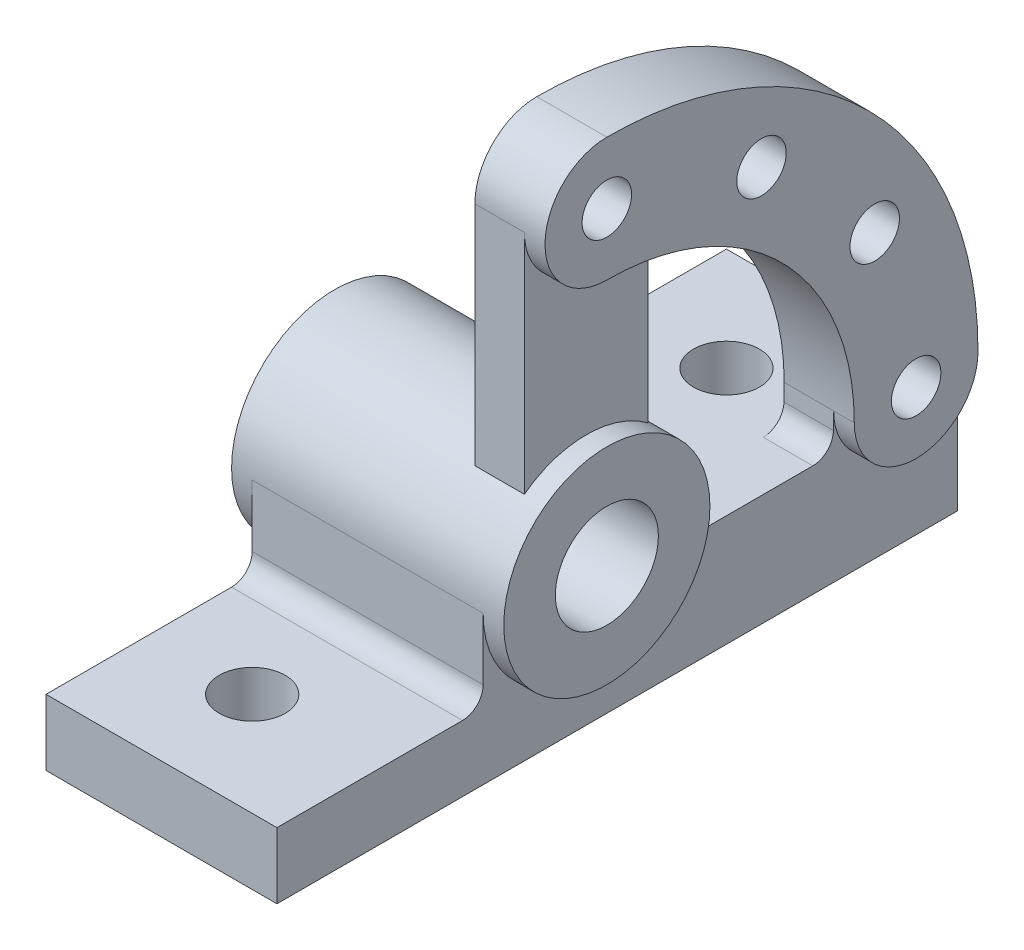
ISO-10303-21;
HEADER;
FILE_DESCRIPTION(('STEP AP214'),'2;1');
FILE_NAME('part.step','',(''),(''),'','','');
FILE_SCHEMA(('AUTOMOTIVE_DESIGN { 1 0 10303 214 1 1 1 1 }'));
ENDSEC;
DATA;
#1=APPLICATION_CONTEXT('core data for automotive mechanical design processes');
#2=APPLICATION_PROTOCOL_DEFINITION('international standard','automotive_design',2000,#1);
#3=PRODUCT_CONTEXT('',#1,'mechanical');
#4=PRODUCT('Part','Part','',(#3));
#5=PRODUCT_RELATED_PRODUCT_CATEGORY('part','',(#4));
#6=PRODUCT_DEFINITION_FORMATION('','',#4);
#7=PRODUCT_DEFINITION_CONTEXT('part definition',#1,'design');
#8=PRODUCT_DEFINITION('design','',#6,#7);
#9=PRODUCT_DEFINITION_SHAPE('','',#8);
#10=(LENGTH_UNIT() NAMED_UNIT(*) SI_UNIT(.MILLI.,.METRE.));
#11=(NAMED_UNIT(*) PLANE_ANGLE_UNIT() SI_UNIT($,.RADIAN.));
#12=(NAMED_UNIT(*) SI_UNIT($,.STERADIAN.) SOLID_ANGLE_UNIT());
#13=UNCERTAINTY_MEASURE_WITH_UNIT(LENGTH_MEASURE(1.E-05),#10,'distance_accuracy_value','');
#14=(GEOMETRIC_REPRESENTATION_CONTEXT(3) GLOBAL_UNCERTAINTY_ASSIGNED_CONTEXT((#13)) GLOBAL_UNIT_ASSIGNED_CONTEXT((#10,
#11,#12)) REPRESENTATION_CONTEXT('',''));
#15=CARTESIAN_POINT('',(0.,0.,0.));
#16=DIRECTION('',(0.,0.,1.));
#17=DIRECTION('',(1.,0.,0.));
#18=AXIS2_PLACEMENT_3D('',#15,#16,#17);
#19=CARTESIAN_POINT('',(-28.,36.,7.50000000000001));
#20=DIRECTION('',(1.,0.,0.));
#21=DIRECTION('',(0.,0.,-1.));
#22=AXIS2_PLACEMENT_3D('',#19,#20,#21);
#23=CYLINDRICAL_SURFACE('',#22,25.);
#24=DIRECTION('',(1.,0.,0.));
#25=VECTOR('',#24,1.);
#26=CARTESIAN_POINT('',(-28.,36.,32.5));
#27=LINE('',#26,#25);
#28=CARTESIAN_POINT('',(-28.,36.,32.5));
#29=VERTEX_POINT('',#28);
#30=CARTESIAN_POINT('',(28.,36.,32.5));
#31=VERTEX_POINT('',#30);
#32=EDGE_CURVE('E338',#29,#31,#27,.T.);
#33=ORIENTED_EDGE('',*,*,#32,.T.);
#34=CARTESIAN_POINT('',(28.,36.,7.5));
#35=DIRECTION('',(1.,0.,0.));
#36=DIRECTION('',(0.,0.,-1.));
#37=AXIS2_PLACEMENT_3D('',#34,#35,#36);
#38=CIRCLE('',#37,25.);
#39=CARTESIAN_POINT('',(28.,32.6666666666667,-17.2767812455308));
#40=VERTEX_POINT('',#39);
#41=EDGE_CURVE('E300',#31,#40,#38,.T.);
#42=ORIENTED_EDGE('',*,*,#41,.T.);
#43=DIRECTION('',(1.,0.,0.));
#44=VECTOR('',#43,1.);
#45=CARTESIAN_POINT('',(-28.,32.6666666666667,-17.2767812455308));
#46=LINE('',#45,#44);
#47=CARTESIAN_POINT('',(-28.,32.6666666666667,-17.2767812455308));
#48=VERTEX_POINT('',#47);
#49=EDGE_CURVE('E343',#48,#40,#46,.T.);
#50=ORIENTED_EDGE('',*,*,#49,.F.);
#51=CARTESIAN_POINT('',(-28.,36.,7.50000000000001));
#52=DIRECTION('',(-1.,0.,0.));
#53=DIRECTION('',(0.,0.,1.));
#54=AXIS2_PLACEMENT_3D('',#51,#52,#53);
#55=CIRCLE('',#54,25.);
#56=EDGE_CURVE('E57',#48,#29,#55,.T.);
#57=ORIENTED_EDGE('',*,*,#56,.T.);
#58=EDGE_LOOP('',(#33,#42,#50,#57));
#59=FACE_BOUND('',#58,.T.);
#60=CARTESIAN_POINT('',(-33.,36.,7.50000000000001));
#61=DIRECTION('',(-1.,0.,0.));
#62=DIRECTION('',(0.,0.,1.));
#63=AXIS2_PLACEMENT_3D('',#60,#61,#62);
#64=CIRCLE('',#63,25.);
#65=CARTESIAN_POINT('',(-33.,36.,32.5));
#66=VERTEX_POINT('',#65);
#67=EDGE_CURVE('E308',#66,#66,#64,.T.);
#68=ORIENTED_EDGE('',*,*,#67,.F.);
#69=EDGE_LOOP('',(#68));
#70=FACE_BOUND('',#69,.T.);
#71=CARTESIAN_POINT('',(33.,36.,7.5));
#72=DIRECTION('',(1.,0.,0.));
#73=DIRECTION('',(0.,0.,-1.));
#74=AXIS2_PLACEMENT_3D('',#71,#72,#73);
#75=CIRCLE('',#74,25.);
#76=CARTESIAN_POINT('',(33.,36.,-17.5));
#77=VERTEX_POINT('',#76);
#78=EDGE_CURVE('E298',#77,#77,#75,.T.);
#79=ORIENTED_EDGE('',*,*,#78,.F.);
#80=EDGE_LOOP('',(#79));
#81=FACE_BOUND('',#80,.T.);
#82=DIRECTION('',(1.,0.,0.));
#83=VECTOR('',#82,1.);
#84=CARTESIAN_POINT('',(-28.,56.,-7.50000000000005));
#85=LINE('',#84,#83);
#86=CARTESIAN_POINT('',(28.,56.,-7.50000000000006));
#87=VERTEX_POINT('',#86);
#88=CARTESIAN_POINT('',(16.,56.,-7.50000000000005));
#89=VERTEX_POINT('',#88);
#90=EDGE_CURVE('E63',#87,#89,#85,.F.);
#91=ORIENTED_EDGE('',*,*,#90,.F.);
#92=CARTESIAN_POINT('',(28.,36.,7.5));
#93=DIRECTION('',(-1.,0.,0.));
#94=DIRECTION('',(0.,0.,1.));
#95=AXIS2_PLACEMENT_3D('',#92,#93,#94);
#96=CIRCLE('',#95,25.);
#97=CARTESIAN_POINT('',(28.,56.,22.4999999999999));
#98=VERTEX_POINT('',#97);
#99=EDGE_CURVE('E70',#87,#98,#96,.F.);
#100=ORIENTED_EDGE('',*,*,#99,.T.);
#101=DIRECTION('',(1.,0.,0.));
#102=VECTOR('',#101,1.);
#103=CARTESIAN_POINT('',(-28.,56.,22.4999999999999));
#104=LINE('',#103,#102);
#105=CARTESIAN_POINT('',(16.,56.,22.4999999999999));
#106=VERTEX_POINT('',#105);
#107=EDGE_CURVE('E179',#106,#98,#104,.T.);
#108=ORIENTED_EDGE('',*,*,#107,.F.);
#109=CARTESIAN_POINT('',(16.,36.,7.50000000000001));
#110=DIRECTION('',(-1.,0.,0.));
#111=DIRECTION('',(0.,0.,1.));
#112=AXIS2_PLACEMENT_3D('',#109,#110,#111);
#113=CIRCLE('',#112,25.);
#114=EDGE_CURVE('E185',#89,#106,#113,.F.);
#115=ORIENTED_EDGE('',*,*,#114,.F.);
#116=EDGE_LOOP('',(#91,#100,#108,#115));
#117=FACE_BOUND('',#116,.T.);
#118=ADVANCED_FACE('F50',(#59,#70,#81,#117),#23,.T.);
#119=CARTESIAN_POINT('',(28.,16.,-82.5));
#120=DIRECTION('',(-1.,0.,0.));
#121=DIRECTION('',(0.,0.,1.));
#122=AXIS2_PLACEMENT_3D('',#119,#120,#121);
#123=PLANE('',#122);
#124=CARTESIAN_POINT('',(28.,36.,-67.5));
#125=DIRECTION('',(1.,0.,0.));
#126=DIRECTION('',(0.,0.,-1.));
#127=AXIS2_PLACEMENT_3D('',#124,#125,#126);
#128=CIRCLE('',#127,15.);
#129=CARTESIAN_POINT('',(28.,36.,-52.5));
#130=VERTEX_POINT('',#129);
#131=CARTESIAN_POINT('',(28.,36.,-82.5));
#132=VERTEX_POINT('',#131);
#133=EDGE_CURVE('E228',#130,#132,#128,.T.);
#134=ORIENTED_EDGE('',*,*,#133,.F.);
#135=DIRECTION('',(0.,-0.999889292581698,0.0148796028331465));
#136=VECTOR('',#135,1.);
#137=CARTESIAN_POINT('',(28.,-0.773122173516407,-51.9527699646989));
#138=LINE('',#137,#136);
#139=CARTESIAN_POINT('',(28.,31.9256019858343,-52.4393678633378));
#140=VERTEX_POINT('',#139);
#141=EDGE_CURVE('E252',#130,#140,#138,.T.);
#142=ORIENTED_EDGE('',*,*,#141,.T.);
#143=CARTESIAN_POINT('',(28.,32.,-47.4399214004293));
#144=DIRECTION('',(1.,0.,0.));
#145=DIRECTION('',(0.,0.,-1.));
#146=AXIS2_PLACEMENT_3D('',#143,#144,#145);
#147=CIRCLE('',#146,4.99999999999999);
#148=CARTESIAN_POINT('',(28.,27.,-47.4399214004293));
#149=VERTEX_POINT('',#148);
#150=EDGE_CURVE('E250',#140,#149,#147,.F.);
#151=ORIENTED_EDGE('',*,*,#150,.T.);
#152=DIRECTION('',(0.,0.,1.));
#153=VECTOR('',#152,1.);
#154=CARTESIAN_POINT('',(28.,27.,0.));
#155=LINE('',#154,#153);
#156=CARTESIAN_POINT('',(28.,27.,-22.232137494637));
#157=VERTEX_POINT('',#156);
#158=EDGE_CURVE('E327',#149,#157,#155,.T.);
#159=ORIENTED_EDGE('',*,*,#158,.T.);
#160=CARTESIAN_POINT('',(28.,32.,-22.232137494637));
#161=DIRECTION('',(1.,0.,0.));
#162=DIRECTION('',(0.,0.,-1.));
#163=AXIS2_PLACEMENT_3D('',#160,#161,#162);
#164=CIRCLE('',#163,5.00000000000001);
#165=EDGE_CURVE('E329',#40,#157,#164,.T.);
#166=ORIENTED_EDGE('',*,*,#165,.F.);
#167=ORIENTED_EDGE('',*,*,#41,.F.);
#168=DIRECTION('',(0.,-1.,0.));
#169=VECTOR('',#168,1.);
#170=CARTESIAN_POINT('',(28.,0.,32.5));
#171=LINE('',#170,#169);
#172=CARTESIAN_POINT('',(28.,21.,32.5));
#173=VERTEX_POINT('',#172);
#174=EDGE_CURVE('E320',#31,#173,#171,.T.);
#175=ORIENTED_EDGE('',*,*,#174,.T.);
#176=CARTESIAN_POINT('',(28.,21.,37.5));
#177=DIRECTION('',(1.,0.,0.));
#178=DIRECTION('',(0.,0.,-1.));
#179=AXIS2_PLACEMENT_3D('',#176,#177,#178);
#180=CIRCLE('',#179,5.);
#181=CARTESIAN_POINT('',(28.,16.,37.5));
#182=VERTEX_POINT('',#181);
#183=EDGE_CURVE('E310',#173,#182,#180,.F.);
#184=ORIENTED_EDGE('',*,*,#183,.T.);
#185=DIRECTION('',(0.,0.,-1.));
#186=VECTOR('',#185,1.);
#187=CARTESIAN_POINT('',(28.,16.,-82.5));
#188=LINE('',#187,#186);
#189=CARTESIAN_POINT('',(28.,16.,82.5));
#190=VERTEX_POINT('',#189);
#191=EDGE_CURVE('E352',#190,#182,#188,.T.);
#192=ORIENTED_EDGE('',*,*,#191,.F.);
#193=DIRECTION('',(0.,-1.,0.));
#194=VECTOR('',#193,1.);
#195=CARTESIAN_POINT('',(28.,16.,82.5));
#196=LINE('',#195,#194);
#197=CARTESIAN_POINT('',(28.,0.,82.5));
#198=VERTEX_POINT('',#197);
#199=EDGE_CURVE('E356',#190,#198,#196,.T.);
#200=ORIENTED_EDGE('',*,*,#199,.T.);
#201=DIRECTION('',(0.,0.,-1.));
#202=VECTOR('',#201,1.);
#203=CARTESIAN_POINT('',(28.,0.,-82.5));
#204=LINE('',#203,#202);
#205=CARTESIAN_POINT('',(28.,0.,-82.5));
#206=VERTEX_POINT('',#205);
#207=EDGE_CURVE('E340',#198,#206,#204,.T.);
#208=ORIENTED_EDGE('',*,*,#207,.T.);
#209=DIRECTION('',(0.,-1.,0.));
#210=VECTOR('',#209,1.);
#211=CARTESIAN_POINT('',(28.,16.,-82.5));
#212=LINE('',#211,#210);
#213=EDGE_CURVE('E315',#132,#206,#212,.T.);
#214=ORIENTED_EDGE('',*,*,#213,.F.);
#215=EDGE_LOOP('',(#134,#142,#151,#159,#166,#167,#175,#184,#192,#200,#208,#214));
#216=FACE_BOUND('',#215,.T.);
#217=ADVANCED_FACE('F47',(#216),#123,.F.);
#218=CARTESIAN_POINT('',(0.,16.,0.));
#219=DIRECTION('',(0.,1.,0.));
#220=DIRECTION('',(0.,0.,1.));
#221=AXIS2_PLACEMENT_3D('',#218,#219,#220);
#222=PLANE('',#221);
#223=CARTESIAN_POINT('',(-2.99999999999999,16.,57.5));
#224=DIRECTION('',(0.,1.,0.));
#225=DIRECTION('',(0.,0.,1.));
#226=AXIS2_PLACEMENT_3D('',#223,#224,#225);
#227=CIRCLE('',#226,8.);
#228=CARTESIAN_POINT('',(-2.99999999999999,16.,65.5));
#229=VERTEX_POINT('',#228);
#230=EDGE_CURVE('E210',#229,#229,#227,.T.);
#231=ORIENTED_EDGE('',*,*,#230,.F.);
#232=EDGE_LOOP('',(#231));
#233=FACE_BOUND('',#232,.T.);
#234=ORIENTED_EDGE('',*,*,#191,.T.);
#235=DIRECTION('',(1.,0.,0.));
#236=VECTOR('',#235,1.);
#237=CARTESIAN_POINT('',(-28.,16.,37.5));
#238=LINE('',#237,#236);
#239=CARTESIAN_POINT('',(-28.,16.,37.5));
#240=VERTEX_POINT('',#239);
#241=EDGE_CURVE('E324',#240,#182,#238,.T.);
#242=ORIENTED_EDGE('',*,*,#241,.F.);
#243=DIRECTION('',(0.,0.,1.));
#244=VECTOR('',#243,1.);
#245=CARTESIAN_POINT('',(-28.,16.,-82.5));
#246=LINE('',#245,#244);
#247=CARTESIAN_POINT('',(-28.,16.,82.5));
#248=VERTEX_POINT('',#247);
#249=EDGE_CURVE('E353',#240,#248,#246,.T.);
#250=ORIENTED_EDGE('',*,*,#249,.T.);
#251=DIRECTION('',(1.,0.,0.));
#252=VECTOR('',#251,1.);
#253=CARTESIAN_POINT('',(-28.,16.,82.5));
#254=LINE('',#253,#252);
#255=EDGE_CURVE('E358',#248,#190,#254,.T.);
#256=ORIENTED_EDGE('',*,*,#255,.T.);
#257=EDGE_LOOP('',(#234,#242,#250,#256));
#258=FACE_BOUND('',#257,.T.);
#259=ADVANCED_FACE('F470',(#233,#258),#222,.T.);
#260=CARTESIAN_POINT('',(-28.,16.,-82.5));
#261=DIRECTION('',(0.,0.,1.));
#262=DIRECTION('',(1.,0.,0.));
#263=AXIS2_PLACEMENT_3D('',#260,#261,#262);
#264=PLANE('',#263);
#265=ORIENTED_EDGE('',*,*,#213,.T.);
#266=DIRECTION('',(-1.,0.,0.));
#267=VECTOR('',#266,1.);
#268=CARTESIAN_POINT('',(-28.,0.,-82.5));
#269=LINE('',#268,#267);
#270=CARTESIAN_POINT('',(-28.,0.,-82.5));
#271=VERTEX_POINT('',#270);
#272=EDGE_CURVE('E363',#206,#271,#269,.T.);
#273=ORIENTED_EDGE('',*,*,#272,.T.);
#274=DIRECTION('',(0.,-1.,0.));
#275=VECTOR('',#274,1.);
#276=CARTESIAN_POINT('',(-28.,16.,-82.5));
#277=LINE('',#276,#275);
#278=CARTESIAN_POINT('',(-28.,27.,-82.5));
#279=VERTEX_POINT('',#278);
#280=EDGE_CURVE('E371',#279,#271,#277,.T.);
#281=ORIENTED_EDGE('',*,*,#280,.F.);
#282=DIRECTION('',(1.,0.,0.));
#283=VECTOR('',#282,1.);
#284=CARTESIAN_POINT('',(-28.,27.,-82.5));
#285=LINE('',#284,#283);
#286=CARTESIAN_POINT('',(16.,27.,-82.5));
#287=VERTEX_POINT('',#286);
#288=EDGE_CURVE('E347',#279,#287,#285,.T.);
#289=ORIENTED_EDGE('',*,*,#288,.T.);
#290=DIRECTION('',(0.,-1.,0.));
#291=VECTOR('',#290,1.);
#292=CARTESIAN_POINT('',(16.,0.,-82.5));
#293=LINE('',#292,#291);
#294=CARTESIAN_POINT('',(16.,36.,-82.5));
#295=VERTEX_POINT('',#294);
#296=EDGE_CURVE('E253',#295,#287,#293,.T.);
#297=ORIENTED_EDGE('',*,*,#296,.F.);
#298=DIRECTION('',(1.,0.,0.));
#299=VECTOR('',#298,1.);
#300=CARTESIAN_POINT('',(16.,36.,-82.5));
#301=LINE('',#300,#299);
#302=EDGE_CURVE('E289',#295,#132,#301,.T.);
#303=ORIENTED_EDGE('',*,*,#302,.T.);
#304=EDGE_LOOP('',(#265,#273,#281,#289,#297,#303));
#305=FACE_BOUND('',#304,.T.);
#306=ADVANCED_FACE('F376',(#305),#264,.F.);
#307=CARTESIAN_POINT('',(-28.,16.,-82.5));
#308=DIRECTION('',(1.,0.,0.));
#309=DIRECTION('',(0.,0.,-1.));
#310=AXIS2_PLACEMENT_3D('',#307,#308,#309);
#311=PLANE('',#310);
#312=ORIENTED_EDGE('',*,*,#56,.F.);
#313=CARTESIAN_POINT('',(-28.,32.,-22.232137494637));
#314=DIRECTION('',(1.,0.,0.));
#315=DIRECTION('',(0.,0.,-1.));
#316=AXIS2_PLACEMENT_3D('',#313,#314,#315);
#317=CIRCLE('',#316,5.00000000000001);
#318=CARTESIAN_POINT('',(-28.,27.,-22.232137494637));
#319=VERTEX_POINT('',#318);
#320=EDGE_CURVE('E319',#48,#319,#317,.T.);
#321=ORIENTED_EDGE('',*,*,#320,.T.);
#322=DIRECTION('',(0.,0.,1.));
#323=VECTOR('',#322,1.);
#324=CARTESIAN_POINT('',(-28.,27.,0.));
#325=LINE('',#324,#323);
#326=EDGE_CURVE('E316',#279,#319,#325,.T.);
#327=ORIENTED_EDGE('',*,*,#326,.F.);
#328=ORIENTED_EDGE('',*,*,#280,.T.);
#329=DIRECTION('',(0.,0.,1.));
#330=VECTOR('',#329,1.);
#331=CARTESIAN_POINT('',(-28.,0.,-82.5));
#332=LINE('',#331,#330);
#333=CARTESIAN_POINT('',(-28.,0.,82.5));
#334=VERTEX_POINT('',#333);
#335=EDGE_CURVE('E361',#271,#334,#332,.T.);
#336=ORIENTED_EDGE('',*,*,#335,.T.);
#337=DIRECTION('',(0.,-1.,0.));
#338=VECTOR('',#337,1.);
#339=CARTESIAN_POINT('',(-28.,16.,82.5));
#340=LINE('',#339,#338);
#341=EDGE_CURVE('E366',#248,#334,#340,.T.);
#342=ORIENTED_EDGE('',*,*,#341,.F.);
#343=ORIENTED_EDGE('',*,*,#249,.F.);
#344=CARTESIAN_POINT('',(-28.,21.,37.5));
#345=DIRECTION('',(1.,0.,0.));
#346=DIRECTION('',(0.,0.,-1.));
#347=AXIS2_PLACEMENT_3D('',#344,#345,#346);
#348=CIRCLE('',#347,5.);
#349=CARTESIAN_POINT('',(-28.,21.,32.5));
#350=VERTEX_POINT('',#349);
#351=EDGE_CURVE('E311',#350,#240,#348,.F.);
#352=ORIENTED_EDGE('',*,*,#351,.F.);
#353=DIRECTION('',(0.,-1.,0.));
#354=VECTOR('',#353,1.);
#355=CARTESIAN_POINT('',(-28.,0.,32.5));
#356=LINE('',#355,#354);
#357=EDGE_CURVE('E325',#29,#350,#356,.T.);
#358=ORIENTED_EDGE('',*,*,#357,.F.);
#359=EDGE_LOOP('',(#312,#321,#327,#328,#336,#342,#343,#352,#358));
#360=FACE_BOUND('',#359,.T.);
#361=ADVANCED_FACE('F395',(#360),#311,.F.);
#362=CARTESIAN_POINT('',(-28.,16.,82.5));
#363=DIRECTION('',(0.,0.,-1.));
#364=DIRECTION('',(-1.,0.,0.));
#365=AXIS2_PLACEMENT_3D('',#362,#363,#364);
#366=PLANE('',#365);
#367=DIRECTION('',(1.,0.,0.));
#368=VECTOR('',#367,1.);
#369=CARTESIAN_POINT('',(-28.,0.,82.5));
#370=LINE('',#369,#368);
#371=EDGE_CURVE('E354',#334,#198,#370,.T.);
#372=ORIENTED_EDGE('',*,*,#371,.T.);
#373=ORIENTED_EDGE('',*,*,#199,.F.);
#374=ORIENTED_EDGE('',*,*,#255,.F.);
#375=ORIENTED_EDGE('',*,*,#341,.T.);
#376=EDGE_LOOP('',(#372,#373,#374,#375));
#377=FACE_BOUND('',#376,.T.);
#378=ADVANCED_FACE('F389',(#377),#366,.F.);
#379=CARTESIAN_POINT('',(0.,0.,0.));
#380=DIRECTION('',(0.,1.,0.));
#381=DIRECTION('',(0.,0.,1.));
#382=AXIS2_PLACEMENT_3D('',#379,#380,#381);
#383=PLANE('',#382);
#384=CARTESIAN_POINT('',(-3.00000000000001,0.,-57.5));
#385=DIRECTION('',(0.,1.,0.));
#386=DIRECTION('',(0.,0.,1.));
#387=AXIS2_PLACEMENT_3D('',#384,#385,#386);
#388=CIRCLE('',#387,8.);
#389=CARTESIAN_POINT('',(-3.00000000000001,0.,-49.5));
#390=VERTEX_POINT('',#389);
#391=EDGE_CURVE('E426',#390,#390,#388,.T.);
#392=ORIENTED_EDGE('',*,*,#391,.T.);
#393=EDGE_LOOP('',(#392));
#394=FACE_BOUND('',#393,.T.);
#395=CARTESIAN_POINT('',(-2.99999999999999,0.,57.5));
#396=DIRECTION('',(0.,1.,0.));
#397=DIRECTION('',(0.,0.,1.));
#398=AXIS2_PLACEMENT_3D('',#395,#396,#397);
#399=CIRCLE('',#398,8.);
#400=CARTESIAN_POINT('',(-2.99999999999999,0.,65.5));
#401=VERTEX_POINT('',#400);
#402=EDGE_CURVE('E51',#401,#401,#399,.T.);
#403=ORIENTED_EDGE('',*,*,#402,.T.);
#404=EDGE_LOOP('',(#403));
#405=FACE_BOUND('',#404,.T.);
#406=ORIENTED_EDGE('',*,*,#207,.F.);
#407=ORIENTED_EDGE('',*,*,#371,.F.);
#408=ORIENTED_EDGE('',*,*,#335,.F.);
#409=ORIENTED_EDGE('',*,*,#272,.F.);
#410=EDGE_LOOP('',(#406,#407,#408,#409));
#411=FACE_BOUND('',#410,.T.);
#412=ADVANCED_FACE('F385',(#394,#405,#411),#383,.F.);
#413=CARTESIAN_POINT('',(-28.,21.,37.5));
#414=DIRECTION('',(1.,0.,0.));
#415=DIRECTION('',(0.,0.,-1.));
#416=AXIS2_PLACEMENT_3D('',#413,#414,#415);
#417=CYLINDRICAL_SURFACE('',#416,5.);
#418=ORIENTED_EDGE('',*,*,#183,.F.);
#419=DIRECTION('',(1.,0.,0.));
#420=VECTOR('',#419,1.);
#421=CARTESIAN_POINT('',(-28.,21.,32.5));
#422=LINE('',#421,#420);
#423=EDGE_CURVE('E333',#350,#173,#422,.T.);
#424=ORIENTED_EDGE('',*,*,#423,.F.);
#425=ORIENTED_EDGE('',*,*,#351,.T.);
#426=ORIENTED_EDGE('',*,*,#241,.T.);
#427=EDGE_LOOP('',(#418,#424,#425,#426));
#428=FACE_BOUND('',#427,.T.);
#429=ADVANCED_FACE('F473',(#428),#417,.F.);
#430=CARTESIAN_POINT('',(-28.,0.,32.5));
#431=DIRECTION('',(0.,0.,1.));
#432=DIRECTION('',(1.,0.,0.));
#433=AXIS2_PLACEMENT_3D('',#430,#431,#432);
#434=PLANE('',#433);
#435=ORIENTED_EDGE('',*,*,#174,.F.);
#436=ORIENTED_EDGE('',*,*,#32,.F.);
#437=ORIENTED_EDGE('',*,*,#357,.T.);
#438=ORIENTED_EDGE('',*,*,#423,.T.);
#439=EDGE_LOOP('',(#435,#436,#437,#438));
#440=FACE_BOUND('',#439,.T.);
#441=ADVANCED_FACE('F454',(#440),#434,.T.);
#442=CARTESIAN_POINT('',(-28.,32.,-22.232137494637));
#443=DIRECTION('',(1.,0.,0.));
#444=DIRECTION('',(0.,0.,-1.));
#445=AXIS2_PLACEMENT_3D('',#442,#443,#444);
#446=CYLINDRICAL_SURFACE('',#445,5.00000000000001);
#447=ORIENTED_EDGE('',*,*,#165,.T.);
#448=DIRECTION('',(1.,0.,0.));
#449=VECTOR('',#448,1.);
#450=CARTESIAN_POINT('',(-28.,27.,-22.232137494637));
#451=LINE('',#450,#449);
#452=EDGE_CURVE('E341',#319,#157,#451,.T.);
#453=ORIENTED_EDGE('',*,*,#452,.F.);
#454=ORIENTED_EDGE('',*,*,#320,.F.);
#455=ORIENTED_EDGE('',*,*,#49,.T.);
#456=EDGE_LOOP('',(#447,#453,#454,#455));
#457=FACE_BOUND('',#456,.T.);
#458=ADVANCED_FACE('F441',(#457),#446,.F.);
#459=CARTESIAN_POINT('',(-28.,27.,0.));
#460=DIRECTION('',(0.,1.,0.));
#461=DIRECTION('',(0.,0.,1.));
#462=AXIS2_PLACEMENT_3D('',#459,#460,#461);
#463=PLANE('',#462);
#464=CARTESIAN_POINT('',(-3.00000000000001,27.,-57.5));
#465=DIRECTION('',(0.,1.,0.));
#466=DIRECTION('',(0.,0.,1.));
#467=AXIS2_PLACEMENT_3D('',#464,#465,#466);
#468=CIRCLE('',#467,8.);
#469=CARTESIAN_POINT('',(-3.00000000000001,27.,-49.5));
#470=VERTEX_POINT('',#469);
#471=EDGE_CURVE('E430',#470,#470,#468,.T.);
#472=ORIENTED_EDGE('',*,*,#471,.F.);
#473=EDGE_LOOP('',(#472));
#474=FACE_BOUND('',#473,.T.);
#475=DIRECTION('',(1.,0.,0.));
#476=VECTOR('',#475,1.);
#477=CARTESIAN_POINT('',(16.,27.,-47.4399214004293));
#478=LINE('',#477,#476);
#479=CARTESIAN_POINT('',(16.,27.,-47.4399214004293));
#480=VERTEX_POINT('',#479);
#481=EDGE_CURVE('E277',#480,#149,#478,.T.);
#482=ORIENTED_EDGE('',*,*,#481,.F.);
#483=DIRECTION('',(0.,0.,-1.));
#484=VECTOR('',#483,1.);
#485=CARTESIAN_POINT('',(16.,27.,0.));
#486=LINE('',#485,#484);
#487=EDGE_CURVE('E11',#480,#287,#486,.T.);
#488=ORIENTED_EDGE('',*,*,#487,.T.);
#489=ORIENTED_EDGE('',*,*,#288,.F.);
#490=ORIENTED_EDGE('',*,*,#326,.T.);
#491=ORIENTED_EDGE('',*,*,#452,.T.);
#492=ORIENTED_EDGE('',*,*,#158,.F.);
#493=EDGE_LOOP('',(#482,#488,#489,#490,#491,#492));
#494=FACE_BOUND('',#493,.T.);
#495=ADVANCED_FACE('F396',(#474,#494),#463,.T.);
#496=CARTESIAN_POINT('',(-28.,36.,7.50000000000001));
#497=DIRECTION('',(1.,0.,0.));
#498=DIRECTION('',(0.,0.,-1.));
#499=AXIS2_PLACEMENT_3D('',#496,#497,#498);
#500=CYLINDRICAL_SURFACE('',#499,12.5);
#501=CARTESIAN_POINT('',(-33.,36.,7.50000000000001));
#502=DIRECTION('',(-1.,0.,0.));
#503=DIRECTION('',(0.,0.,1.));
#504=AXIS2_PLACEMENT_3D('',#501,#502,#503);
#505=CIRCLE('',#504,12.5);
#506=CARTESIAN_POINT('',(-33.,36.,20.));
#507=VERTEX_POINT('',#506);
#508=EDGE_CURVE('E303',#507,#507,#505,.T.);
#509=ORIENTED_EDGE('',*,*,#508,.T.);
#510=EDGE_LOOP('',(#509));
#511=FACE_BOUND('',#510,.T.);
#512=CARTESIAN_POINT('',(33.,36.,7.5));
#513=DIRECTION('',(1.,0.,0.));
#514=DIRECTION('',(0.,0.,-1.));
#515=AXIS2_PLACEMENT_3D('',#512,#513,#514);
#516=CIRCLE('',#515,12.5);
#517=CARTESIAN_POINT('',(33.,36.,-4.99999999999999));
#518=VERTEX_POINT('',#517);
#519=EDGE_CURVE('E285',#518,#518,#516,.T.);
#520=ORIENTED_EDGE('',*,*,#519,.T.);
#521=EDGE_LOOP('',(#520));
#522=FACE_BOUND('',#521,.T.);
#523=ADVANCED_FACE('F444',(#511,#522),#500,.F.);
#524=CARTESIAN_POINT('',(-33.,36.,7.50000000000001));
#525=DIRECTION('',(-1.,0.,0.));
#526=DIRECTION('',(0.,0.,1.));
#527=AXIS2_PLACEMENT_3D('',#524,#525,#526);
#528=PLANE('',#527);
#529=ORIENTED_EDGE('',*,*,#67,.T.);
#530=EDGE_LOOP('',(#529));
#531=FACE_BOUND('',#530,.T.);
#532=ORIENTED_EDGE('',*,*,#508,.F.);
#533=EDGE_LOOP('',(#532));
#534=FACE_BOUND('',#533,.T.);
#535=ADVANCED_FACE('F453',(#531,#534),#528,.T.);
#536=CARTESIAN_POINT('',(33.,36.,7.5));
#537=DIRECTION('',(1.,0.,0.));
#538=DIRECTION('',(0.,0.,-1.));
#539=AXIS2_PLACEMENT_3D('',#536,#537,#538);
#540=PLANE('',#539);
#541=ORIENTED_EDGE('',*,*,#78,.T.);
#542=EDGE_LOOP('',(#541));
#543=FACE_BOUND('',#542,.T.);
#544=ORIENTED_EDGE('',*,*,#519,.F.);
#545=EDGE_LOOP('',(#544));
#546=FACE_BOUND('',#545,.T.);
#547=ADVANCED_FACE('F478',(#543,#546),#540,.T.);
#548=CARTESIAN_POINT('',(16.,32.,-47.4399214004293));
#549=DIRECTION('',(1.,0.,0.));
#550=DIRECTION('',(0.,0.,-1.));
#551=AXIS2_PLACEMENT_3D('',#548,#549,#550);
#552=CYLINDRICAL_SURFACE('',#551,4.99999999999999);
#553=ORIENTED_EDGE('',*,*,#150,.F.);
#554=DIRECTION('',(1.,0.,0.));
#555=VECTOR('',#554,1.);
#556=CARTESIAN_POINT('',(16.,31.9256019858343,-52.4393678633378));
#557=LINE('',#556,#555);
#558=CARTESIAN_POINT('',(16.,31.9256019858343,-52.4393678633378));
#559=VERTEX_POINT('',#558);
#560=EDGE_CURVE('E278',#559,#140,#557,.T.);
#561=ORIENTED_EDGE('',*,*,#560,.F.);
#562=CARTESIAN_POINT('',(16.,32.,-47.4399214004293));
#563=DIRECTION('',(1.,0.,0.));
#564=DIRECTION('',(0.,0.,-1.));
#565=AXIS2_PLACEMENT_3D('',#562,#563,#564);
#566=CIRCLE('',#565,4.99999999999999);
#567=EDGE_CURVE('E246',#559,#480,#566,.F.);
#568=ORIENTED_EDGE('',*,*,#567,.T.);
#569=ORIENTED_EDGE('',*,*,#481,.T.);
#570=EDGE_LOOP('',(#553,#561,#568,#569));
#571=FACE_BOUND('',#570,.T.);
#572=ADVANCED_FACE('F403',(#571),#552,.F.);
#573=CARTESIAN_POINT('',(16.,-0.773122173516407,-51.9527699646989));
#574=DIRECTION('',(0.,0.0148796028331465,0.999889292581698));
#575=DIRECTION('',(0.,-0.999889292581698,0.0148796028331465));
#576=AXIS2_PLACEMENT_3D('',#573,#574,#575);
#577=PLANE('',#576);
#578=ORIENTED_EDGE('',*,*,#141,.F.);
#579=DIRECTION('',(1.,0.,0.));
#580=VECTOR('',#579,1.);
#581=CARTESIAN_POINT('',(16.,36.,-52.5));
#582=LINE('',#581,#580);
#583=CARTESIAN_POINT('',(16.,36.,-52.5));
#584=VERTEX_POINT('',#583);
#585=EDGE_CURVE('E283',#584,#130,#582,.T.);
#586=ORIENTED_EDGE('',*,*,#585,.F.);
#587=DIRECTION('',(0.,-0.999889292581698,0.0148796028331465));
#588=VECTOR('',#587,1.);
#589=CARTESIAN_POINT('',(16.,-0.773122173516407,-51.9527699646989));
#590=LINE('',#589,#588);
#591=EDGE_CURVE('E261',#584,#559,#590,.T.);
#592=ORIENTED_EDGE('',*,*,#591,.T.);
#593=ORIENTED_EDGE('',*,*,#560,.T.);
#594=EDGE_LOOP('',(#578,#586,#592,#593));
#595=FACE_BOUND('',#594,.T.);
#596=ADVANCED_FACE('F408',(#595),#577,.T.);
#597=CARTESIAN_POINT('',(16.,36.,7.50000000000001));
#598=DIRECTION('',(1.,0.,0.));
#599=DIRECTION('',(0.,0.,-1.));
#600=AXIS2_PLACEMENT_3D('',#597,#598,#599);
#601=CYLINDRICAL_SURFACE('',#600,60.);
#602=CARTESIAN_POINT('',(28.,35.9999999999994,7.50000000000059));
#603=DIRECTION('',(-1.,0.,0.));
#604=DIRECTION('',(0.,0.,1.));
#605=AXIS2_PLACEMENT_3D('',#602,#603,#604);
#606=CIRCLE('',#605,60.0000000000006);
#607=CARTESIAN_POINT('',(28.,96.,7.5));
#608=VERTEX_POINT('',#607);
#609=CARTESIAN_POINT('',(28.,94.0947501931113,-7.49999999999997));
#610=VERTEX_POINT('',#609);
#611=EDGE_CURVE('E416',#608,#610,#606,.T.);
#612=ORIENTED_EDGE('',*,*,#611,.T.);
#613=DIRECTION('',(-1.,0.,0.));
#614=VECTOR('',#613,1.);
#615=CARTESIAN_POINT('',(28.,94.0947501931111,-7.49999999999997));
#616=LINE('',#615,#614);
#617=CARTESIAN_POINT('',(16.,94.0947501931113,-7.5));
#618=VERTEX_POINT('',#617);
#619=EDGE_CURVE('E190',#610,#618,#616,.T.);
#620=ORIENTED_EDGE('',*,*,#619,.T.);
#621=CARTESIAN_POINT('',(16.,36.,7.50000000000001));
#622=DIRECTION('',(1.,0.,0.));
#623=DIRECTION('',(0.,0.,-1.));
#624=AXIS2_PLACEMENT_3D('',#621,#622,#623);
#625=CIRCLE('',#624,60.);
#626=EDGE_CURVE('E259',#584,#618,#625,.T.);
#627=ORIENTED_EDGE('',*,*,#626,.F.);
#628=ORIENTED_EDGE('',*,*,#585,.T.);
#629=DIRECTION('',(-1.,0.,0.));
#630=VECTOR('',#629,1.);
#631=CARTESIAN_POINT('',(33.,36.,-52.5));
#632=LINE('',#631,#630);
#633=CARTESIAN_POINT('',(33.,36.,-52.5));
#634=VERTEX_POINT('',#633);
#635=EDGE_CURVE('E244',#634,#130,#632,.T.);
#636=ORIENTED_EDGE('',*,*,#635,.F.);
#637=CARTESIAN_POINT('',(33.,35.9999999999997,7.50000000000029));
#638=DIRECTION('',(-1.,0.,0.));
#639=DIRECTION('',(0.,0.,1.));
#640=AXIS2_PLACEMENT_3D('',#637,#638,#639);
#641=CIRCLE('',#640,60.0000000000003);
#642=CARTESIAN_POINT('',(33.,96.,7.5));
#643=VERTEX_POINT('',#642);
#644=EDGE_CURVE('E234',#643,#634,#641,.T.);
#645=ORIENTED_EDGE('',*,*,#644,.F.);
#646=DIRECTION('',(1.,0.,0.));
#647=VECTOR('',#646,1.);
#648=CARTESIAN_POINT('',(16.,96.,7.50000000000001));
#649=LINE('',#648,#647);
#650=EDGE_CURVE('E288',#608,#643,#649,.T.);
#651=ORIENTED_EDGE('',*,*,#650,.F.);
#652=EDGE_LOOP('',(#612,#620,#627,#628,#636,#645,#651));
#653=FACE_BOUND('',#652,.T.);
#654=ADVANCED_FACE('F491',(#653),#601,.F.);
#655=CARTESIAN_POINT('',(16.,111.,7.50000000000001));
#656=DIRECTION('',(1.,0.,0.));
#657=DIRECTION('',(0.,0.,-1.));
#658=AXIS2_PLACEMENT_3D('',#655,#656,#657);
#659=CYLINDRICAL_SURFACE('',#658,15.);
#660=DIRECTION('',(-1.,0.,0.));
#661=VECTOR('',#660,1.);
#662=CARTESIAN_POINT('',(28.,111.,22.5));
#663=LINE('',#662,#661);
#664=CARTESIAN_POINT('',(28.,111.,22.5));
#665=VERTEX_POINT('',#664);
#666=CARTESIAN_POINT('',(16.,111.,22.5));
#667=VERTEX_POINT('',#666);
#668=EDGE_CURVE('E205',#665,#667,#663,.T.);
#669=ORIENTED_EDGE('',*,*,#668,.F.);
#670=CARTESIAN_POINT('',(28.,111.,7.50000000000004));
#671=DIRECTION('',(1.,0.,0.));
#672=DIRECTION('',(0.,0.,-1.));
#673=AXIS2_PLACEMENT_3D('',#670,#671,#672);
#674=CIRCLE('',#673,15.);
#675=EDGE_CURVE('E420',#665,#608,#674,.T.);
#676=ORIENTED_EDGE('',*,*,#675,.T.);
#677=ORIENTED_EDGE('',*,*,#650,.T.);
#678=CARTESIAN_POINT('',(33.,111.,7.50000000000003));
#679=DIRECTION('',(1.,0.,0.));
#680=DIRECTION('',(0.,0.,-1.));
#681=AXIS2_PLACEMENT_3D('',#678,#679,#680);
#682=CIRCLE('',#681,15.);
#683=CARTESIAN_POINT('',(33.,126.,7.50000000000005));
#684=VERTEX_POINT('',#683);
#685=EDGE_CURVE('E235',#684,#643,#682,.T.);
#686=ORIENTED_EDGE('',*,*,#685,.F.);
#687=DIRECTION('',(1.,0.,0.));
#688=VECTOR('',#687,1.);
#689=CARTESIAN_POINT('',(16.,126.,7.50000000000001));
#690=LINE('',#689,#688);
#691=CARTESIAN_POINT('',(16.,126.,7.50000000000001));
#692=VERTEX_POINT('',#691);
#693=EDGE_CURVE('E286',#692,#684,#690,.T.);
#694=ORIENTED_EDGE('',*,*,#693,.F.);
#695=CARTESIAN_POINT('',(16.,111.,7.50000000000001));
#696=DIRECTION('',(1.,0.,0.));
#697=DIRECTION('',(0.,0.,-1.));
#698=AXIS2_PLACEMENT_3D('',#695,#696,#697);
#699=CIRCLE('',#698,15.);
#700=EDGE_CURVE('E260',#692,#667,#699,.T.);
#701=ORIENTED_EDGE('',*,*,#700,.T.);
#702=EDGE_LOOP('',(#669,#676,#677,#686,#694,#701));
#703=FACE_BOUND('',#702,.T.);
#704=ADVANCED_FACE('F490',(#703),#659,.T.);
#705=CARTESIAN_POINT('',(16.,36.,7.50000000000001));
#706=DIRECTION('',(1.,0.,0.));
#707=DIRECTION('',(0.,0.,-1.));
#708=AXIS2_PLACEMENT_3D('',#705,#706,#707);
#709=CYLINDRICAL_SURFACE('',#708,90.);
#710=ORIENTED_EDGE('',*,*,#693,.T.);
#711=CARTESIAN_POINT('',(33.,35.9999999999996,7.50000000000032));
#712=DIRECTION('',(1.,0.,0.));
#713=DIRECTION('',(0.,0.,1.));
#714=AXIS2_PLACEMENT_3D('',#711,#712,#713);
#715=CIRCLE('',#714,90.0000000000003);
#716=CARTESIAN_POINT('',(33.,36.,-82.5));
#717=VERTEX_POINT('',#716);
#718=EDGE_CURVE('E229',#717,#684,#715,.T.);
#719=ORIENTED_EDGE('',*,*,#718,.F.);
#720=DIRECTION('',(-1.,0.,0.));
#721=VECTOR('',#720,1.);
#722=CARTESIAN_POINT('',(33.,36.,-82.5));
#723=LINE('',#722,#721);
#724=EDGE_CURVE('E239',#717,#132,#723,.T.);
#725=ORIENTED_EDGE('',*,*,#724,.T.);
#726=ORIENTED_EDGE('',*,*,#302,.F.);
#727=CARTESIAN_POINT('',(16.,36.,7.50000000000001));
#728=DIRECTION('',(1.,0.,0.));
#729=DIRECTION('',(0.,0.,-1.));
#730=AXIS2_PLACEMENT_3D('',#727,#728,#729);
#731=CIRCLE('',#730,90.);
#732=EDGE_CURVE('E255',#295,#692,#731,.T.);
#733=ORIENTED_EDGE('',*,*,#732,.T.);
#734=EDGE_LOOP('',(#710,#719,#725,#726,#733));
#735=FACE_BOUND('',#734,.T.);
#736=ADVANCED_FACE('F483',(#735),#709,.T.);
#737=CARTESIAN_POINT('',(16.,111.,7.50000000000001));
#738=DIRECTION('',(1.,0.,0.));
#739=DIRECTION('',(0.,0.,-1.));
#740=AXIS2_PLACEMENT_3D('',#737,#738,#739);
#741=CYLINDRICAL_SURFACE('',#740,6.);
#742=CARTESIAN_POINT('',(16.,111.,7.50000000000001));
#743=DIRECTION('',(1.,0.,0.));
#744=DIRECTION('',(0.,0.,-1.));
#745=AXIS2_PLACEMENT_3D('',#742,#743,#744);
#746=CIRCLE('',#745,6.);
#747=CARTESIAN_POINT('',(16.,111.,1.5));
#748=VERTEX_POINT('',#747);
#749=EDGE_CURVE('E269',#748,#748,#746,.T.);
#750=ORIENTED_EDGE('',*,*,#749,.F.);
#751=EDGE_LOOP('',(#750));
#752=FACE_BOUND('',#751,.T.);
#753=CARTESIAN_POINT('',(33.,111.,7.50000000000003));
#754=DIRECTION('',(1.,0.,0.));
#755=DIRECTION('',(0.,0.,-1.));
#756=AXIS2_PLACEMENT_3D('',#753,#754,#755);
#757=CIRCLE('',#756,6.00000000000003);
#758=CARTESIAN_POINT('',(33.,111.,1.5));
#759=VERTEX_POINT('',#758);
#760=EDGE_CURVE('E223',#759,#759,#757,.T.);
#761=ORIENTED_EDGE('',*,*,#760,.T.);
#762=EDGE_LOOP('',(#761));
#763=FACE_BOUND('',#762,.T.);
#764=ADVANCED_FACE('F486',(#752,#763),#741,.F.);
#765=CARTESIAN_POINT('',(16.,73.5000000000001,-57.4519052838328));
#766=DIRECTION('',(1.,0.,0.));
#767=DIRECTION('',(0.,0.,-1.));
#768=AXIS2_PLACEMENT_3D('',#765,#766,#767);
#769=CYLINDRICAL_SURFACE('',#768,6.);
#770=CARTESIAN_POINT('',(16.,73.5000000000001,-57.4519052838328));
#771=DIRECTION('',(1.,0.,0.));
#772=DIRECTION('',(0.,0.,-1.));
#773=AXIS2_PLACEMENT_3D('',#770,#771,#772);
#774=CIRCLE('',#773,6.);
#775=CARTESIAN_POINT('',(16.,73.5000000000001,-63.4519052838328));
#776=VERTEX_POINT('',#775);
#777=EDGE_CURVE('E270',#776,#776,#774,.T.);
#778=ORIENTED_EDGE('',*,*,#777,.F.);
#779=EDGE_LOOP('',(#778));
#780=FACE_BOUND('',#779,.T.);
#781=CARTESIAN_POINT('',(33.,73.5000000000001,-57.4519052838328));
#782=DIRECTION('',(1.,0.,0.));
#783=DIRECTION('',(0.,0.,-1.));
#784=AXIS2_PLACEMENT_3D('',#781,#782,#783);
#785=CIRCLE('',#784,6.);
#786=CARTESIAN_POINT('',(33.,73.5000000000001,-63.4519052838328));
#787=VERTEX_POINT('',#786);
#788=EDGE_CURVE('E218',#787,#787,#785,.T.);
#789=ORIENTED_EDGE('',*,*,#788,.T.);
#790=EDGE_LOOP('',(#789));
#791=FACE_BOUND('',#790,.T.);
#792=ADVANCED_FACE('F502',(#780,#791),#769,.F.);
#793=CARTESIAN_POINT('',(16.,100.951905283833,-29.9999999999998));
#794=DIRECTION('',(1.,0.,0.));
#795=DIRECTION('',(0.,0.,-1.));
#796=AXIS2_PLACEMENT_3D('',#793,#794,#795);
#797=CYLINDRICAL_SURFACE('',#796,6.00000000000001);
#798=CARTESIAN_POINT('',(16.,100.951905283833,-29.9999999999998));
#799=DIRECTION('',(1.,0.,0.));
#800=DIRECTION('',(0.,0.,-1.));
#801=AXIS2_PLACEMENT_3D('',#798,#799,#800);
#802=CIRCLE('',#801,6.00000000000001);
#803=CARTESIAN_POINT('',(16.,100.951905283833,-35.9999999999998));
#804=VERTEX_POINT('',#803);
#805=EDGE_CURVE('E262',#804,#804,#802,.T.);
#806=ORIENTED_EDGE('',*,*,#805,.F.);
#807=EDGE_LOOP('',(#806));
#808=FACE_BOUND('',#807,.T.);
#809=CARTESIAN_POINT('',(33.,100.951905283833,-29.9999999999998));
#810=DIRECTION('',(1.,0.,0.));
#811=DIRECTION('',(0.,0.,-1.));
#812=AXIS2_PLACEMENT_3D('',#809,#810,#811);
#813=CIRCLE('',#812,6.00000000000001);
#814=CARTESIAN_POINT('',(33.,100.951905283833,-35.9999999999998));
#815=VERTEX_POINT('',#814);
#816=EDGE_CURVE('E225',#815,#815,#813,.T.);
#817=ORIENTED_EDGE('',*,*,#816,.T.);
#818=EDGE_LOOP('',(#817));
#819=FACE_BOUND('',#818,.T.);
#820=ADVANCED_FACE('F500',(#808,#819),#797,.F.);
#821=CARTESIAN_POINT('',(16.,36.,-67.5));
#822=DIRECTION('',(1.,0.,0.));
#823=DIRECTION('',(0.,0.,-1.));
#824=AXIS2_PLACEMENT_3D('',#821,#822,#823);
#825=CYLINDRICAL_SURFACE('',#824,6.);
#826=CARTESIAN_POINT('',(16.,36.,-67.5));
#827=DIRECTION('',(1.,0.,0.));
#828=DIRECTION('',(0.,0.,-1.));
#829=AXIS2_PLACEMENT_3D('',#826,#827,#828);
#830=CIRCLE('',#829,6.);
#831=CARTESIAN_POINT('',(16.,36.,-73.5));
#832=VERTEX_POINT('',#831);
#833=EDGE_CURVE('E272',#832,#832,#830,.T.);
#834=ORIENTED_EDGE('',*,*,#833,.F.);
#835=EDGE_LOOP('',(#834));
#836=FACE_BOUND('',#835,.T.);
#837=CARTESIAN_POINT('',(33.,36.,-67.5));
#838=DIRECTION('',(1.,0.,0.));
#839=DIRECTION('',(0.,0.,-1.));
#840=AXIS2_PLACEMENT_3D('',#837,#838,#839);
#841=CIRCLE('',#840,6.);
#842=CARTESIAN_POINT('',(33.,36.,-73.5));
#843=VERTEX_POINT('',#842);
#844=EDGE_CURVE('E216',#843,#843,#841,.T.);
#845=ORIENTED_EDGE('',*,*,#844,.T.);
#846=EDGE_LOOP('',(#845));
#847=FACE_BOUND('',#846,.T.);
#848=ADVANCED_FACE('F498',(#836,#847),#825,.F.);
#849=CARTESIAN_POINT('',(16.,0.,0.));
#850=DIRECTION('',(1.,0.,0.));
#851=DIRECTION('',(0.,0.,-1.));
#852=AXIS2_PLACEMENT_3D('',#849,#850,#851);
#853=PLANE('',#852);
#854=ORIENTED_EDGE('',*,*,#626,.T.);
#855=DIRECTION('',(0.,-1.,0.));
#856=VECTOR('',#855,1.);
#857=CARTESIAN_POINT('',(16.,94.0947501931111,-7.49999999999997));
#858=LINE('',#857,#856);
#859=EDGE_CURVE('E200',#618,#89,#858,.T.);
#860=ORIENTED_EDGE('',*,*,#859,.T.);
#861=ORIENTED_EDGE('',*,*,#114,.T.);
#862=DIRECTION('',(0.,1.,0.));
#863=VECTOR('',#862,1.);
#864=CARTESIAN_POINT('',(16.,111.,22.5));
#865=LINE('',#864,#863);
#866=EDGE_CURVE('E198',#106,#667,#865,.T.);
#867=ORIENTED_EDGE('',*,*,#866,.T.);
#868=ORIENTED_EDGE('',*,*,#700,.F.);
#869=ORIENTED_EDGE('',*,*,#732,.F.);
#870=ORIENTED_EDGE('',*,*,#296,.T.);
#871=ORIENTED_EDGE('',*,*,#487,.F.);
#872=ORIENTED_EDGE('',*,*,#567,.F.);
#873=ORIENTED_EDGE('',*,*,#591,.F.);
#874=EDGE_LOOP('',(#854,#860,#861,#867,#868,#869,#870,#871,#872,#873));
#875=FACE_BOUND('',#874,.T.);
#876=ORIENTED_EDGE('',*,*,#805,.T.);
#877=EDGE_LOOP('',(#876));
#878=FACE_BOUND('',#877,.T.);
#879=ORIENTED_EDGE('',*,*,#777,.T.);
#880=EDGE_LOOP('',(#879));
#881=FACE_BOUND('',#880,.T.);
#882=ORIENTED_EDGE('',*,*,#749,.T.);
#883=EDGE_LOOP('',(#882));
#884=FACE_BOUND('',#883,.T.);
#885=ORIENTED_EDGE('',*,*,#833,.T.);
#886=EDGE_LOOP('',(#885));
#887=FACE_BOUND('',#886,.T.);
#888=ADVANCED_FACE('F191',(#875,#878,#881,#884,#887),#853,.F.);
#889=CARTESIAN_POINT('',(33.,35.9999999999998,-29.9999999999998));
#890=DIRECTION('',(-1.,0.,0.));
#891=DIRECTION('',(0.,0.,1.));
#892=AXIS2_PLACEMENT_3D('',#889,#890,#891);
#893=PLANE('',#892);
#894=ORIENTED_EDGE('',*,*,#718,.T.);
#895=ORIENTED_EDGE('',*,*,#685,.T.);
#896=ORIENTED_EDGE('',*,*,#644,.T.);
#897=CARTESIAN_POINT('',(33.,36.,-67.5));
#898=DIRECTION('',(1.,0.,0.));
#899=DIRECTION('',(0.,0.,-1.));
#900=AXIS2_PLACEMENT_3D('',#897,#898,#899);
#901=CIRCLE('',#900,15.);
#902=EDGE_CURVE('E240',#634,#717,#901,.T.);
#903=ORIENTED_EDGE('',*,*,#902,.T.);
#904=EDGE_LOOP('',(#894,#895,#896,#903));
#905=FACE_BOUND('',#904,.T.);
#906=ORIENTED_EDGE('',*,*,#760,.F.);
#907=EDGE_LOOP('',(#906));
#908=FACE_BOUND('',#907,.T.);
#909=ORIENTED_EDGE('',*,*,#816,.F.);
#910=EDGE_LOOP('',(#909));
#911=FACE_BOUND('',#910,.T.);
#912=ORIENTED_EDGE('',*,*,#788,.F.);
#913=EDGE_LOOP('',(#912));
#914=FACE_BOUND('',#913,.T.);
#915=ORIENTED_EDGE('',*,*,#844,.F.);
#916=EDGE_LOOP('',(#915));
#917=FACE_BOUND('',#916,.T.);
#918=ADVANCED_FACE('F514',(#905,#908,#911,#914,#917),#893,.F.);
#919=CARTESIAN_POINT('',(33.,36.,-67.5));
#920=DIRECTION('',(-1.,0.,0.));
#921=DIRECTION('',(0.,0.,1.));
#922=AXIS2_PLACEMENT_3D('',#919,#920,#921);
#923=CYLINDRICAL_SURFACE('',#922,15.);
#924=ORIENTED_EDGE('',*,*,#133,.T.);
#925=ORIENTED_EDGE('',*,*,#724,.F.);
#926=ORIENTED_EDGE('',*,*,#902,.F.);
#927=ORIENTED_EDGE('',*,*,#635,.T.);
#928=EDGE_LOOP('',(#924,#925,#926,#927));
#929=FACE_BOUND('',#928,.T.);
#930=ADVANCED_FACE('F513',(#929),#923,.T.);
#931=CARTESIAN_POINT('',(28.,94.0947501931111,-7.49999999999997));
#932=DIRECTION('',(0.,0.,-1.));
#933=DIRECTION('',(0.,1.,0.));
#934=AXIS2_PLACEMENT_3D('',#931,#932,#933);
#935=PLANE('',#934);
#936=DIRECTION('',(0.,-1.,0.));
#937=VECTOR('',#936,1.);
#938=CARTESIAN_POINT('',(28.,94.0947501931111,-7.49999999999997));
#939=LINE('',#938,#937);
#940=EDGE_CURVE('E207',#610,#87,#939,.T.);
#941=ORIENTED_EDGE('',*,*,#940,.T.);
#942=ORIENTED_EDGE('',*,*,#90,.T.);
#943=ORIENTED_EDGE('',*,*,#859,.F.);
#944=ORIENTED_EDGE('',*,*,#619,.F.);
#945=EDGE_LOOP('',(#941,#942,#943,#944));
#946=FACE_BOUND('',#945,.T.);
#947=ADVANCED_FACE('F412',(#946),#935,.T.);
#948=CARTESIAN_POINT('',(28.,111.,22.5));
#949=DIRECTION('',(0.,0.,1.));
#950=DIRECTION('',(0.,-1.,0.));
#951=AXIS2_PLACEMENT_3D('',#948,#949,#950);
#952=PLANE('',#951);
#953=ORIENTED_EDGE('',*,*,#866,.F.);
#954=ORIENTED_EDGE('',*,*,#107,.T.);
#955=DIRECTION('',(0.,1.,0.));
#956=VECTOR('',#955,1.);
#957=CARTESIAN_POINT('',(28.,111.,22.5));
#958=LINE('',#957,#956);
#959=EDGE_CURVE('E204',#98,#665,#958,.T.);
#960=ORIENTED_EDGE('',*,*,#959,.T.);
#961=ORIENTED_EDGE('',*,*,#668,.T.);
#962=EDGE_LOOP('',(#953,#954,#960,#961));
#963=FACE_BOUND('',#962,.T.);
#964=ADVANCED_FACE('F203',(#963),#952,.T.);
#965=CARTESIAN_POINT('',(28.,35.9999999999994,7.50000000000059));
#966=DIRECTION('',(-1.,0.,0.));
#967=DIRECTION('',(0.,0.,1.));
#968=AXIS2_PLACEMENT_3D('',#965,#966,#967);
#969=PLANE('',#968);
#970=ORIENTED_EDGE('',*,*,#99,.F.);
#971=ORIENTED_EDGE('',*,*,#940,.F.);
#972=ORIENTED_EDGE('',*,*,#611,.F.);
#973=ORIENTED_EDGE('',*,*,#675,.F.);
#974=ORIENTED_EDGE('',*,*,#959,.F.);
#975=EDGE_LOOP('',(#970,#971,#972,#973,#974));
#976=FACE_BOUND('',#975,.T.);
#977=ADVANCED_FACE('F521',(#976),#969,.F.);
#978=CARTESIAN_POINT('',(-2.99999999999999,-4.,57.5));
#979=DIRECTION('',(0.,1.,0.));
#980=DIRECTION('',(0.,0.,1.));
#981=AXIS2_PLACEMENT_3D('',#978,#979,#980);
#982=CYLINDRICAL_SURFACE('',#981,8.);
#983=ORIENTED_EDGE('',*,*,#230,.T.);
#984=EDGE_LOOP('',(#983));
#985=FACE_BOUND('',#984,.T.);
#986=ORIENTED_EDGE('',*,*,#402,.F.);
#987=EDGE_LOOP('',(#986));
#988=FACE_BOUND('',#987,.T.);
#989=ADVANCED_FACE('F437',(#985,#988),#982,.F.);
#990=CARTESIAN_POINT('',(-3.00000000000001,0.,-57.5));
#991=DIRECTION('',(0.,1.,0.));
#992=DIRECTION('',(0.,0.,1.));
#993=AXIS2_PLACEMENT_3D('',#990,#991,#992);
#994=CYLINDRICAL_SURFACE('',#993,8.);
#995=ORIENTED_EDGE('',*,*,#391,.F.);
#996=EDGE_LOOP('',(#995));
#997=FACE_BOUND('',#996,.T.);
#998=ORIENTED_EDGE('',*,*,#471,.T.);
#999=EDGE_LOOP('',(#998));
#1000=FACE_BOUND('',#999,.T.);
#1001=ADVANCED_FACE('F434',(#997,#1000),#994,.F.);
#1002=CLOSED_SHELL('',(#118,#217,#259,#306,#361,#378,#412,#429,#441,#458,#495,#523,#535,#547,
#572,#596,#654,#704,#736,#764,#792,#820,#848,#888,#918,#930,#947,#964,#977,#989,#1001));
#1003=MANIFOLD_SOLID_BREP('B2',#1002);
#1004=ADVANCED_BREP_SHAPE_REPRESENTATION('',(#18,#1003),#14);
#1005=SHAPE_DEFINITION_REPRESENTATION(#9,#1004);
ENDSEC;
END-ISO-10303-21;
